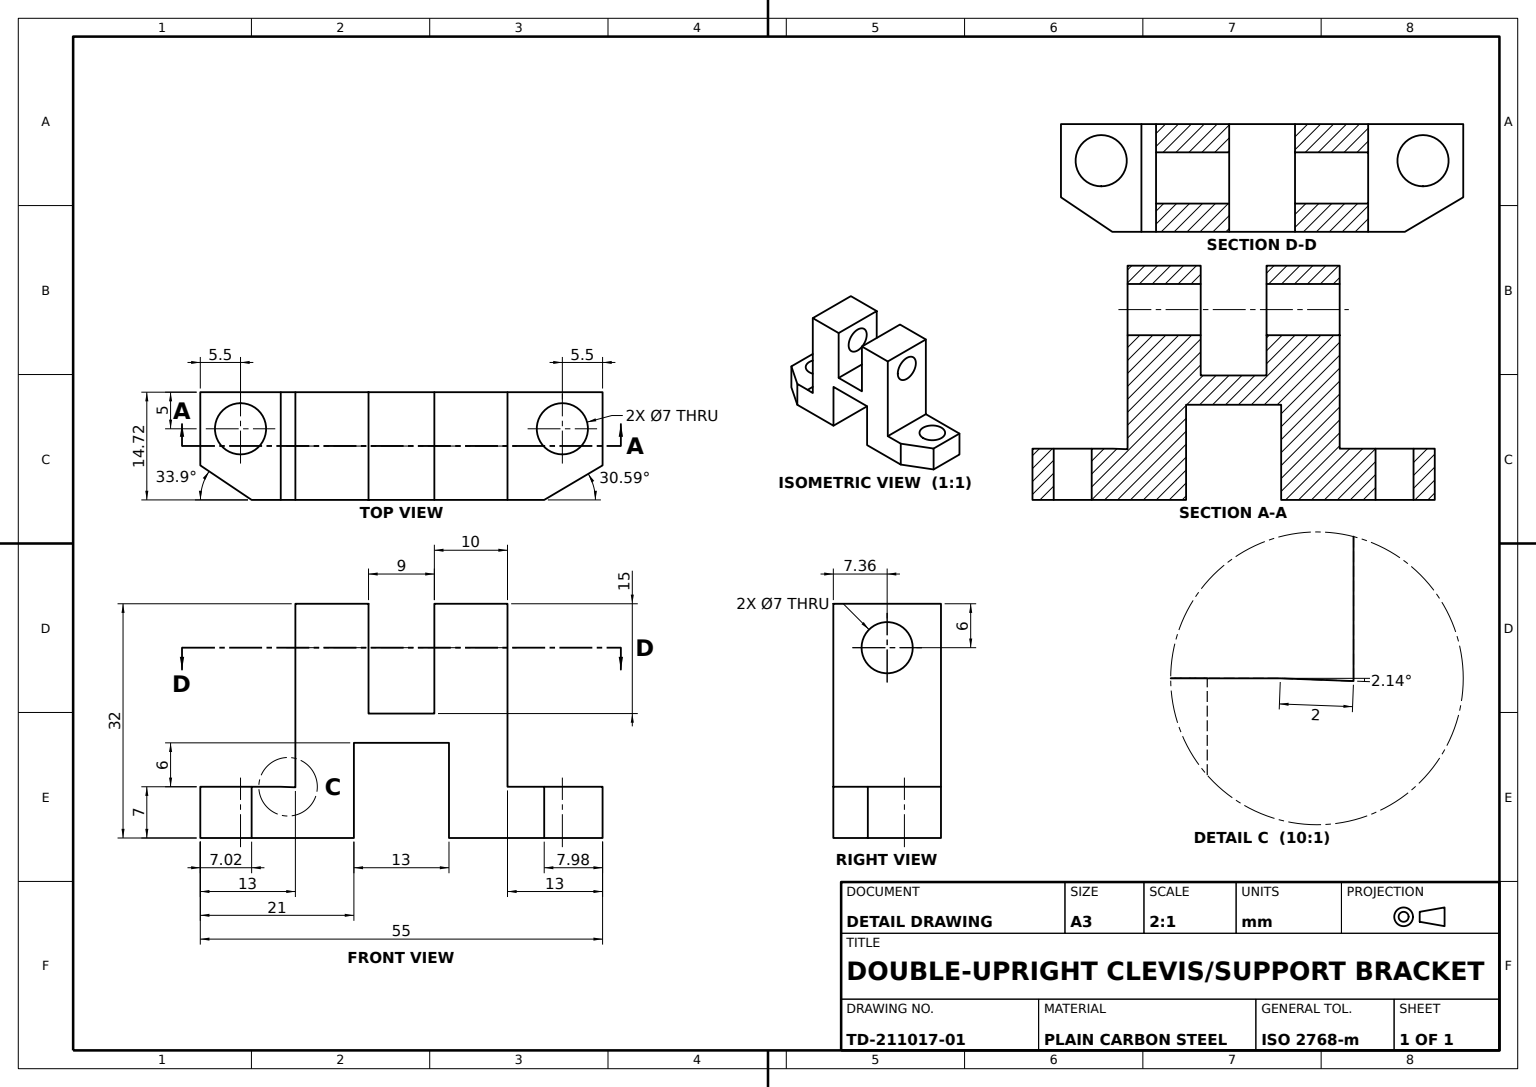
SolidWorks part; units mm, degrees
material "Plain Carbon Steel"
ref_plane "Front Plane" through (0, 0, 0) normal (0, 0, 1) x (1, 0, 0)
ref_plane "Top Plane" through (0, 0, 0) normal (0, 1, 0) x (1, 0, 0)
ref_plane "Right Plane" through (0, 0, 0) normal (1, 0, 0) x (0, 0, -1)
sketch "Base Plate Sketch" plane through (0, 0, 0) normal (0, 1, 0) x (1, 0, 0)
  line L0 (-27.5, 8) -> (-27.5, -2)
  line L1 (-20.481, -6.7172) -> (19.519, -6.7172)
  line L2 (-27.5, -2) -> (-27.5, 8)
  line L3 (-27.5, 8) -> (27.5, 8)
  line L4 (27.5, -2) -> (27.5, 8)
  line L5 (-21.2692, -6.1874) -> (27.5, 8) construction
  line L6 (-27.5, 8) -> (20.697, -6.0209) construction
  line L7 (-27.5, -2) -> (-20.481, -6.7172)
  line L8 (19.519, -6.7172) -> (27.5, -2)
  point P0 (0, 0)
  dimension "D1" = 55
  dimension "D2" = 27.5
  dimension "D3" = 10
  dimension "D4" = 7.019
  dimension "D5" = 47.019
  dimension "D6" = 10
  dimension "D7" = 4.7172
  dimension "D8" = 6.7172
extrude "Base Plate 55x7" add sketch "Base Plate Sketch" along normal mid plane 7 contours L1 L8 L4 L3 L0 L7
sketch "Front Notch Sketch" plane through (0, 0, 6.7172) normal (0, 0, 1) x (1, 0, 0)
  line L1 (-6.5, 4.4294) -> (6.5, 4.4294)
  line L2 (-6.5, 4.4294) -> (-6.5, -4.983)
  line L3 (-6.5, -4.983) -> (6.5, -4.983)
  line L4 (6.5, 4.4294) -> (6.5, -4.983)
  line L5 (-20.481, -3.5) -> (19.519, -3.5) construction
  dimension "D1" = 13
  dimension "D2" = 6.5
  dimension "D3" = 7.9294
  dimension "D4" = 1.483
extrude "Front Notch 13x6.5" cut sketch "Front Notch Sketch" against normal through all
sketch "Upright A Sketch" plane through (0, 0, 6.7172) normal (0, 0, 1) x (1, 0, 0)
  line L0 (-6.5, -3.5) -> (-6.5, 28.5)
  line L1 (-6.5, 28.5) -> (-16.5, 28.5)
  line L2 (-16.5, 28.5) -> (-16.5, -3.5)
  line L3 (-20.481, -3.5) -> (-6.5, -3.5) construction
  line L4 (-16.5, -3.5) -> (-6.5, -3.5)
  dimension "D1" = 10
  dimension "D2" = 32
extrude "Upright A 10x32" add sketch "Upright A Sketch" against normal up to vertex (14.7172 mm away) up to point (-6.5, 3.5, -8)
sketch "Upright B Sketch" plane through (0, 0, 6.7172) normal (0, 0, 1) x (1, 0, 0)
  line L1 (6.5, -3.5) -> (16.5, -3.5)
  line L2 (6.5, -3.5) -> (6.5, 28.5)
  line L3 (6.5, 28.5) -> (16.5, 28.5)
  line L4 (16.5, -3.5) -> (16.5, 28.5)
  dimension "D1" = 10
  dimension "D2" = 32
extrude "Upright B 10x32" add sketch "Upright B Sketch" against normal up to vertex (14.7172 mm away) up to point (6.5, 3.5, -8)
sketch "Upright A Hole Sketch" plane through (0, 3.5, 0) normal (0, 1, 0) x (1, 0, 0)
  line L3 (0, -8.0944) -> (0, 8.0944) construction
  line L5 (-27.5, 3) -> (-16.5, 3) construction
  line L6 (-27.5, 8) -> (-27.5, -2) construction
  line L7 (-16.5, 8) -> (-16.5, -6.7172) construction
  circle A0 centre (-22, 3) radius 3.5
  circle A1 centre (22, 3) radius 3.5
  dimension "D1" = 7
extrude "Upright A Hole" cut sketch "Upright A Hole Sketch" against normal through all
sketch "Infill Boss Sketch" plane through (0, 0, 6.7172) normal (0, 0, 1) x (1, 0, 0)
  line L3 (-6.5, 28.5) -> (6.5, 28.5)
  line L8 (-6.5, 28.5) -> (-6.5, -3.5)
  line L9 (-6.5, -3.5) -> (6.5, -3.5)
  line L10 (6.5, 28.5) -> (6.5, -3.5)
extrude "Infill Boss" add sketch "Infill Boss Sketch" against normal through all
sketch "Rear Notch Sketch" plane through (0, 0, 6.7172) normal (0, 0, 1) x (1, 0, 0)
  line L0 (-20.481, -3.5) -> (19.519, -3.5) construction
  line L1 (-6.5, 9.5) -> (6.5, 9.5)
  line L2 (-6.5, 9.5) -> (-6.5, -3.5)
  line L3 (-6.5, -3.5) -> (6.5, -3.5)
  line L4 (6.5, 9.5) -> (6.5, -3.5)
  dimension "D1" = 13
  dimension "D2" = 6.5
  dimension "D3" = 13
extrude "Rear Notch 13x6.5" cut sketch "Rear Notch Sketch" against normal through all
sketch "Slot Cut Sketch" plane through (0, 0, 6.7172) normal (0, 0, 1) x (1, 0, 0)
  line L0 (0, 28.5) -> (0, -3.944) construction
  line L1 (16.5, 28.5) -> (-16.5, 28.5) construction
  line L3 (-4.5, 28.5) -> (4.5, 28.5)
  line L4 (-4.5, 28.5) -> (-4.5, 13.5)
  line L5 (-4.5, 13.5) -> (4.5, 13.5)
  line L6 (4.5, 28.5) -> (4.5, 13.5)
  dimension "D1" = 9
  dimension "D2" = 4.5
  dimension "D3" = 15
extrude "Slot Cut" cut sketch "Slot Cut Sketch" against normal through all
sketch "Upright B Hole Sketch" plane through (16.5, 0, 0) normal (1, 0, 0) x (0, 0, -1)
  line L0 (8, 28.5) -> (-6.7172, 28.5) construction
  line L1 (-6.7172, 3.5) -> (-6.7172, 28.5) construction
  circle A0 centre (0.6414, 22.5) radius 3.5
  dimension "D1" = 7
  dimension "D2" = 6
  dimension "D3" = 7.3586
extrude "Upright B Hole" cut sketch "Upright B Hole Sketch" against normal through all
sketch "Flange Profile Cut A Sketch" plane through (0, 0, 6.7172) normal (0, 0, 1) x (1, 0, 0)
  line L0 (4.5, 28.5) -> (14.5, 28.5)
  line L1 (16.5, 28.5) -> (4.5, 28.5) construction
  line L2 (14.5, 28.5) -> (14.5, 3.5)
  line L3 (14.5, 3.5) -> (16.5, 3.5)
  line L4 (16.5, 3.5) -> (19.519, 3.5) construction
  line L5 (14.5, 28.5) -> (16.5, 28.5)
  line L6 (16.5, 28.5) -> (16.5, 3.5)
  line L7 (16.5, 3.5) -> (16.5, 28.5) construction
  line M16 (16.5, 3.5) -> (16.5, 28.5)
  line M17 (16.5, 28.5) -> (4.5, 28.5)
  dimension "D1" = 10
extrude "Flange Profile Cut A" cut sketch "Flange Profile Cut A Sketch" against normal through all contours L2 L3 M16 M17
sketch "Flange Profile Cut B Sketch" plane through (0, 0, 6.7172) normal (0, 0, 1) x (1, 0, 0)
  line L0 (-4.5, 28.5) -> (-14.5, 28.5)
  line L1 (-4.5, 28.5) -> (-16.5, 28.5) construction
  line L2 (-14.5, 28.5) -> (-14.5, 3.4254)
  line L3 (-14.5, 3.4254) -> (-16.5, 3.5)
  line L4 (-16.5, 3.5) -> (-16.5, 28.5)
  line L5 (-16.5, 28.5) -> (-14.5, 28.5)
  line M8 (-4.5, 28.5) -> (-16.5, 28.5)
  line M9 (-16.5, 28.5) -> (-16.5, 3.5)
  dimension "D1" = 10
  dimension "D2" = 25.0746
extrude "Flange Profile Cut B" cut sketch "Flange Profile Cut B Sketch" against normal through all contours L3 L2 M8 M9
